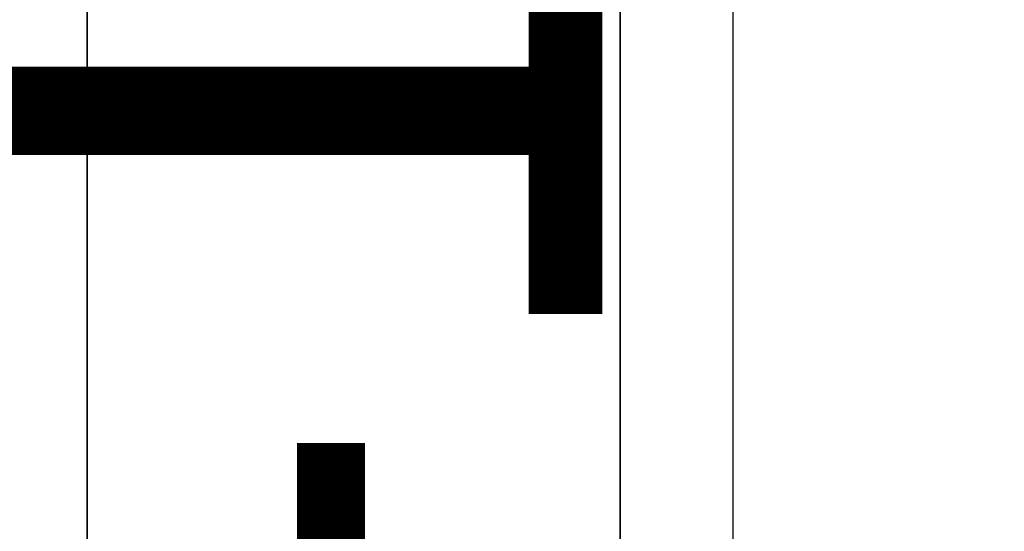
# Model space of a CAD drawing. Units: inches. Extents: x 2083 to 3317, y 1141 to 2115.
# Tile 76 of 256: x 2225.82 to 2242.45, y 1485.75 to 1494.39. Entities that reach past the tile are written whole.
import ezdxf

# ---------------------------------------------------------------- set-up
doc = ezdxf.new("R2010")
doc.units = ezdxf.units.IN
doc.layers.add('A-ANNO-DIMS', color=2, linetype='Continuous', lineweight=18)
doc.layers.add('A-WALL', color=7, linetype='Continuous', lineweight=35)
doc.layers.add('A-WALL-PATT', color=251, linetype='Continuous', lineweight=13, true_color=0x636466)
doc.styles.get("Standard").update_dxf_attribs({"font": 'arial.ttf'})
doc.dimstyles.new('ISO-25', dxfattribs={"dimtxt": 12, "dimasz": 12, "dimexe": 1.25, "dimexo": 0.625, "dimtad": 1, "dimlunit": 3, "dimtxsty": 'Standard', "dimcen": 2.5, "dimadec": 0, "dimazin": 0, "dimtfac": 1, "dimtmove": 0, "dimatfit": 3, "dimfxl": 1, "dimarcsym": 0})

# ---------------------------------------------------------------- blocks, each defined once
blk = doc.blocks.new('*D30')
at = {"layer": 'A-ANNO-DIMS', "color": 0, "lineweight": -2, "transparency": 16777216}
for p, q in [((2240.018, 1445.274), (2240.018, 1448.046)), ((2254.329, 1445.274), (2254.329, 1448.046)), ((2228.018, 1446.796), (2216.018, 1446.796)), ((2240.018, 1446.796), (2254.329, 1446.796)), ((2266.329, 1446.796), (2413.765, 1446.796))]:
    blk.add_line(p, q, dxfattribs=at)
at = {"layer": 'A-ANNO-DIMS', "color": 0, "transparency": 16777216}
for points in [[(2228.018, 1448.796), (2228.018, 1444.796), (2240.018, 1446.796)], [(2266.329, 1448.796), (2266.329, 1444.796), (2254.329, 1446.796)]]:
    blk.add_solid(points, dxfattribs=at)
at = {"layer": 'Defpoints', "color": 0, "transparency": 16777216}
for p in [(2254.329, 1446.796), (2240.018, 1444.649), (2254.329, 1444.649)]:
    blk.add_point(p, dxfattribs=at)
at = {"layer": 'A-ANNO-DIMS', "color": 0, "transparency": 16777216, "insert": (2346.047, 1453.625), "char_height": 12, "attachment_point": 5}
blk.add_mtext('WC 1\'-2 1/2" TYP.', dxfattribs=at)
blk = doc.blocks.new('*D31')
at = {"layer": 'A-ANNO-DIMS', "color": 0, "lineweight": -2, "transparency": 16777216}
for p, q in [((2237.871, 1456.649), (2237.871, 1541.915)), ((2239.393, 1444.649), (2236.621, 1444.649)), ((2237.871, 1431.548), (2237.871, 1444.649)), ((2239.393, 1431.548), (2236.621, 1431.548)), ((2237.871, 1419.548), (2237.871, 1407.548))]:
    blk.add_line(p, q, dxfattribs=at)
at = {"layer": 'A-ANNO-DIMS', "color": 0, "transparency": 16777216}
for points in [[(2235.871, 1456.649), (2239.871, 1456.649), (2237.871, 1444.649)], [(2235.871, 1419.548), (2239.871, 1419.548), (2237.871, 1431.548)]]:
    blk.add_solid(points, dxfattribs=at)
at = {"layer": 'Defpoints', "color": 0, "transparency": 16777216}
for p in [(2237.871, 1444.649), (2240.018, 1444.649), (2240.018, 1431.548)]:
    blk.add_point(p, dxfattribs=at)
at = {"layer": 'A-ANNO-DIMS', "color": 0, "transparency": 16777216, "insert": (2231.217, 1505.282), "char_height": 12, "attachment_point": 5, "rotation": 90}
blk.add_mtext('1\'-1" TYP.', dxfattribs=at)
blk = doc.blocks.new('*D45')
at = {"layer": 'A-ANNO-DIMS', "color": 0, "lineweight": -2, "transparency": 16777216}
for p, q in [((2235.96, 1478.386), (2235.96, 1531.361)), ((2418.96, 1478.386), (2418.96, 1531.361)), ((2247.96, 1530.111), (2406.96, 1530.111))]:
    blk.add_line(p, q, dxfattribs=at)
at = {"layer": 'A-ANNO-DIMS', "color": 0, "transparency": 16777216}
for points in [[(2247.96, 1532.111), (2247.96, 1528.111), (2235.96, 1530.111)], [(2406.96, 1532.111), (2406.96, 1528.111), (2418.96, 1530.111)]]:
    blk.add_solid(points, dxfattribs=at)
at = {"layer": 'Defpoints', "color": 0, "transparency": 16777216}
for p in [(2418.96, 1530.111), (2235.96, 1477.761), (2418.96, 1477.761)]:
    blk.add_point(p, dxfattribs=at)
at = {"layer": 'A-ANNO-DIMS', "color": 0, "transparency": 16777216, "insert": (2327.46, 1536.867), "char_height": 12, "attachment_point": 5}
blk.add_mtext('15\'-3"', dxfattribs=at)
blk = doc.blocks.new('*D62')
at = {"layer": 'A-ANNO-DIMS', "color": 0, "lineweight": -2, "transparency": 16777216}
for p, q in [((2235.96, 1469.386), (2235.96, 1522.361)), ((2379.96, 1469.386), (2379.96, 1522.361)), ((2247.96, 1521.111), (2367.96, 1521.111))]:
    blk.add_line(p, q, dxfattribs=at)
at = {"layer": 'A-ANNO-DIMS', "color": 0, "transparency": 16777216}
for points in [[(2247.96, 1523.111), (2247.96, 1519.111), (2235.96, 1521.111)], [(2367.96, 1523.111), (2367.96, 1519.111), (2379.96, 1521.111)]]:
    blk.add_solid(points, dxfattribs=at)
at = {"layer": 'Defpoints', "color": 0, "transparency": 16777216}
for p in [(2379.96, 1521.111), (2235.96, 1468.761), (2379.96, 1468.761)]:
    blk.add_point(p, dxfattribs=at)
at = {"layer": 'A-ANNO-DIMS', "color": 0, "transparency": 16777216, "insert": (2307.96, 1527.863), "char_height": 12, "attachment_point": 5}
blk.add_mtext('12\'-0"', dxfattribs=at)
blk = doc.blocks.new('*D64')
at = {"layer": 'A-ANNO-DIMS', "color": 0, "lineweight": -2, "transparency": 16777216}
for p, q in [((2236.585, 1702.761), (2289.56, 1702.761)), ((2288.31, 1690.761), (2288.31, 1489.761)), ((2236.585, 1477.761), (2289.56, 1477.761))]:
    blk.add_line(p, q, dxfattribs=at)
at = {"layer": 'A-ANNO-DIMS', "color": 0, "transparency": 16777216}
for points in [[(2286.31, 1690.761), (2290.31, 1690.761), (2288.31, 1702.761)], [(2286.31, 1489.761), (2290.31, 1489.761), (2288.31, 1477.761)]]:
    blk.add_solid(points, dxfattribs=at)
at = {"layer": 'Defpoints', "color": 0, "transparency": 16777216}
for p in [(2235.96, 1702.761), (2235.96, 1477.761), (2288.31, 1477.761)]:
    blk.add_point(p, dxfattribs=at)
at = {"layer": 'A-ANNO-DIMS', "color": 0, "transparency": 16777216, "insert": (2281.558, 1590.261), "char_height": 12, "attachment_point": 5, "rotation": 90}
blk.add_mtext('18\'-9"', dxfattribs=at)

msp = doc.modelspace()

# ---------------------------------------------------------------- hatches: boundary and pattern name
at = {"layer": 'A-WALL-PATT'}
h = msp.add_hatch(color=256, dxfattribs=at)
h.dxf.hatch_style = 1
h.paths.add_polyline_path([(3126.96, 2020.761), (2748.96, 2020.761), (2604.96, 2020.761), (2226.96, 2020.761), (2226.96, 1702.761), (2466.96, 1702.761), (2466.96, 1582.761), (2418.96, 1582.761), (2418.96, 1477.761), (2226.96, 1477.761), (2226.96, 1263.261), (2544.96, 1263.261), (2544.96, 1411.761), (2604.96, 1411.761), (2685.96, 1411.761), (2685.96, 1420.761), (2604.96, 1420.761), (2604.96, 1573.761), (2604.96, 1702.761), (2604.96, 2011.761), (2748.96, 2011.761), (2748.96, 1702.761), (2862.96, 1702.761), (2862.96, 1621.761), (2871.96, 1621.761), (2871.96, 1702.761), (2883.96, 1702.761), (2883.96, 1706.939, -0.026459), (2883.96, 1711.761), (2757.96, 1711.761), (2757.96, 1807.761), (2787.96, 1807.761), (2787.96, 1812.261), (2757.96, 1812.261), (2757.96, 2011.761), (2877.96, 2011.761), (2877.96, 1812.261), (2847.96, 1812.261), (2847.96, 1807.761), (2889.836, 1807.761), (2889.836, 1812.261), (2882.46, 1812.261), (2882.46, 2011.761), (3117.96, 2011.761), (3117.96, 1812.261), (2937.836, 1812.261), (2937.836, 1807.761), (2995.71, 1807.761), (2995.71, 1796.118), (3000.21, 1796.118), (3000.21, 1807.761), (3117.96, 1807.761), (3117.96, 1711.761), (3000.21, 1711.761), (3000.21, 1760.118), (2998.573, 1760.118, -0.020711), (2995.71, 1760.118), (2995.71, 1711.761), (2931.96, 1711.761), (2931.96, 1702.761), (3126.96, 1702.761)])
h.paths.add_polyline_path([(2471.46, 2011.761), (2471.46, 1810.011), (2462.717, 1810.011), (2462.717, 1805.511), (2505.96, 1805.511), (2505.96, 1810.011), (2475.96, 1810.011), (2475.96, 2011.761), (2595.96, 2011.761), (2595.96, 1810.011), (2565.96, 1810.011), (2565.96, 1805.511), (2595.96, 1805.511), (2595.96, 1711.761), (2235.96, 1711.761), (2235.96, 1805.511), (2353.71, 1805.511), (2353.71, 1796.054), (2358.21, 1796.054), (2358.21, 1805.511), (2414.717, 1805.511), (2414.717, 1810.011), (2235.96, 1810.011), (2235.96, 2011.761)], flags=16)
h.paths.add_polyline_path([(2270.205, 1994.61), (2270.205, 1970.61), (2246.205, 1970.61), (2246.205, 1994.61)], flags=0)
edge = h.paths.add_edge_path(flags=0)
edge.add_ellipse((2332.027, 1899.798), major_axis=(-3.043, 3.043), ratio=0.168252, start_angle=-161.3322, end_angle=-156.3071, ccw=False)
edge.add_ellipse((2333.082, 1898.744), major_axis=(-1.055, 1.055), ratio=0.453532, start_angle=-123.371, end_angle=-94.1591)
edge = h.paths.add_edge_path(flags=0)
edge.add_ellipse((2332.027, 1968.876), major_axis=(3.043, 3.043), ratio=0.168252, start_angle=18.6678, end_angle=23.6929)
edge.add_spline(control_points=[(2332.926, 1970.691), (2332.227, 1970.336), (2330.894, 1969.659), (2328.413, 1970.932), (2327.204, 1967.749), (2324.71, 1969.956), (2322.533, 1967.012), (2320.013, 1971.296), (2317.68, 1968.158), (2316.041, 1967.102), (2315.427, 1966.81)], knot_values=[0, 0, 0, 0, 2.267059, 4.324559, 6.685584, 8.878641, 11.121502, 14.300359, 17.755284, 19.732645, 19.732645, 19.732645, 19.732645], degree=3, periodic=0)
edge.add_ellipse((2332.027, 1968.876), major_axis=(3.043, 3.043), ratio=0.168252, start_angle=18.6678, end_angle=23.6929, ccw=False)
edge.add_ellipse((2333.082, 1969.931), major_axis=(1.055, 1.055), ratio=0.453532, start_angle=56.629, end_angle=85.8409, ccw=False)
edge = h.paths.add_edge_path(flags=0)
edge.add_spline(control_points=[(2296.428, 1967.988), (2293.628, 1965.336), (2287.704, 1959.727), (2299.744, 1949.996), (2294.533, 1935.669), (2290.573, 1920.604), (2293.394, 1909.974), (2296.185, 1904.967)], knot_values=[0.099185, 0.099185, 0.099185, 0.099185, 0.345301, 0.619822, 0.982653, 1.386093, 1.810555, 1.810555, 1.810555, 1.810555], degree=3, periodic=0)
edge.add_spline(control_points=[(2296.185, 1904.967), (2297.384, 1902.619), (2298.001, 1901.949), (2298.553, 1901.468)], knot_values=[0.006246, 0.006246, 0.006246, 0.006246, 0.055476, 0.055476, 0.055476, 0.055476], degree=3, periodic=0)
edge.add_spline(control_points=[(2298.553, 1901.468), (2297.259, 1900.923), (2295.225, 1900.232), (2293.06, 1900.614), (2292.101, 1900.788), (2292.09, 1900.791)], knot_values=[0.312835, 0.312835, 0.312835, 0.312835, 0.40178, 0.474987, 0.475903, 0.475903, 0.475903, 0.475903], degree=3, periodic=0)
edge.add_arc((2292.794, 1904.664), 3.937, 215.4209, 259.6982, ccw=False)
edge.add_spline(control_points=[(2289.585, 1902.382), (2289.477, 1902.535), (2289.368, 1902.688), (2289.261, 1902.841)], knot_values=[0.102872, 0.102872, 0.102872, 0.102872, 0.116896, 0.116896, 0.116896, 0.116896], degree=3, periodic=0)
edge.add_spline(control_points=[(2289.261, 1902.841), (2288.687, 1902.55), (2287.64, 1902.02), (2285.881, 1901.874), (2283.853, 1901.504), (2281.72, 1899.711), (2278.467, 1899.493), (2276.157, 1901.883), (2272.259, 1899.804), (2267.778, 1901.843), (2262.244, 1900.184), (2257.415, 1901.782), (2254.318, 1900.726), (2253.178, 1900.337)], knot_values=[0, 0, 0, 0, 1.907977, 3.477176, 5.261074, 7.972851, 11.680248, 13.717921, 16.939592, 22.789562, 27.502503, 33.595215, 37.145618, 37.145618, 37.145618, 37.145618], degree=3, periodic=0)
edge.add_line((2253.178, 1900.337), (2250.244, 1902.841))
edge.add_line((2250.244, 1902.841), (2250.244, 1965.833))
edge.add_line((2250.244, 1965.833), (2253.178, 1968.337))
edge.add_spline(control_points=[(2253.178, 1968.337), (2254.318, 1967.948), (2257.415, 1966.892), (2262.244, 1968.49), (2267.778, 1966.831), (2271.527, 1968.537), (2273.876, 1967.828), (2274.207, 1967.728)], knot_values=[0, 0, 0, 0, 0.09018, 0.244935, 0.364644, 0.513233, 0.537855, 0.537855, 0.537855, 0.537855], degree=3, periodic=0)
edge.add_arc((2274.353, 1963.793), 3.937, 72.0511, 92.1279, ccw=False)
edge.add_arc((2281.297, 1985.23), 18.596, 252.0511, 288.5657)
edge.add_arc((2292.317, 1956.029), 12.646, 71.0268, 113.7782, ccw=False)
edge = h.paths.add_edge_path(flags=0)
edge.add_spline(control_points=[(2274.899, 1951.856), (2275.066, 1951.617), (2275.233, 1951.377), (2275.398, 1951.136)], knot_values=[1.409916, 1.409916, 1.409916, 1.409916, 1.43159, 1.43159, 1.43159, 1.43159], degree=3, periodic=0)
edge.add_spline(control_points=[(2275.398, 1951.136), (2275.792, 1950.562), (2276.179, 1949.984), (2276.546, 1949.397)], knot_values=[1.358238, 1.358238, 1.358238, 1.358238, 1.409916, 1.409916, 1.409916, 1.409916], degree=3, periodic=0)
edge.add_line((2276.546, 1949.397), (2277.437, 1947.862))
edge.add_spline(control_points=[(2277.437, 1947.862), (2276.304, 1945.673), (2274.64, 1942.427), (2274.632, 1938.094), (2272.799, 1930.852), (2274.356, 1943.897), (2275.948, 1947.923), (2276.546, 1949.397)], knot_values=[0.005632, 0.005632, 0.005632, 0.005632, 0.186014, 0.266002, 0.357087, 0.59639, 0.739732, 0.739732, 0.739732, 0.739732], degree=3, periodic=0)
edge.add_spline(control_points=[(2276.546, 1949.397), (2276.179, 1949.984), (2275.792, 1950.562), (2275.398, 1951.136)], knot_values=[1.358238, 1.358238, 1.358238, 1.358238, 1.409916, 1.409916, 1.409916, 1.409916], degree=3, periodic=0)
edge.add_spline(control_points=[(2275.398, 1951.136), (2274.943, 1950.08), (2274.208, 1948.025), (2273.935, 1944.851), (2272.469, 1937.627), (2273.466, 1945.696), (2274.701, 1951.059), (2274.899, 1951.856)], knot_values=[0.104364, 0.104364, 0.104364, 0.104364, 0.189636, 0.269624, 0.36071, 0.600013, 0.644622, 0.644622, 0.644622, 0.644622], degree=3, periodic=0)
h.paths.add_polyline_path([(2269.168, 1963.128, -0.357527), (2268.171, 1960.976, -0.092561), (2268.171, 1939.436, -0.357527), (2269.168, 1937.285, -0.357527), (2267.016, 1938.282, -0.164785), (2254.686, 1938.282, -0.357527), (2252.534, 1937.285, -0.357527), (2253.531, 1939.436, -0.092561), (2253.531, 1960.976, -0.357527), (2252.534, 1963.128, -0.357527), (2254.686, 1962.131, -0.164785), (2267.016, 1962.131, -0.357527)], flags=0)
h.paths.add_polyline_path([(2248.874, 1967.802), (2248.874, 1957.028), (2249.458, 1957.028), (2249.458, 1911.647), (2248.874, 1911.647), (2248.874, 1900.873), (2246.512, 1900.873, 0.197327), (2244.15, 1902.457), (2244.15, 1966.218, 0.197327), (2246.512, 1967.802)], flags=0)
h.paths.add_polyline_path([(2269.168, 1931.389, -0.357527), (2268.171, 1929.238, -0.092561), (2268.171, 1907.698, -0.357527), (2269.168, 1905.547, -0.357527), (2267.016, 1906.544, -0.164785), (2254.686, 1906.544, -0.357527), (2252.534, 1905.547, -0.357527), (2253.531, 1907.698, -0.092561), (2253.531, 1929.238, -0.357527), (2252.534, 1931.389, -0.357527), (2254.686, 1930.392, -0.164785), (2267.016, 1930.392, -0.357527)], flags=0)
edge = h.paths.add_edge_path(flags=0)
edge.add_spline(control_points=[(2276.197, 1906.724), (2276.168, 1909.029), (2276.114, 1913.372), (2270.598, 1924.925), (2273.905, 1919.013), (2275.922, 1916.262), (2275.475, 1912.402), (2277.258, 1910.381), (2276.696, 1908.225), (2276.646, 1906.813), (2276.618, 1906.008)], knot_values=[0, 0, 0, 0, 8.61026, 16.221274, 18.843057, 23.804898, 27.440828, 29.356102, 31.203478, 33.650687, 33.650687, 33.650687, 33.650687], degree=3, periodic=0)
edge.add_spline(control_points=[(2276.618, 1906.008), (2276.623, 1905.624), (2276.498, 1904.629), (2275.442, 1903.855), (2274.937, 1903.08), (2274.859, 1902.841)], knot_values=[0.156488, 0.156488, 0.156488, 0.156488, 0.184398, 0.231376, 0.250598, 0.250598, 0.250598, 0.250598], degree=3, periodic=0)
edge.add_line((2274.859, 1902.841), (2276.506, 1902.841))
edge.add_spline(control_points=[(2276.506, 1902.841), (2276.788, 1903.085), (2277.665, 1904.125), (2278.25, 1904.341), (2277.654, 1908.527), (2278.156, 1906.228), (2278.1, 1905.286), (2278.847, 1904.069), (2277.857, 1903.415), (2277.874, 1902.991), (2277.904, 1902.841)], knot_values=[0.059574, 0.059574, 0.059574, 0.059574, 0.080753, 0.103741, 0.16972, 0.176036, 0.207137, 0.240474, 0.262341, 0.27366, 0.27366, 0.27366, 0.27366], degree=3, periodic=0)
edge.add_line((2277.904, 1902.841), (2280.03, 1902.841))
edge.add_spline(control_points=[(2280.03, 1902.841), (2279.888, 1903.088), (2279.499, 1903.982), (2280.152, 1905.939), (2278.104, 1909.658), (2279.762, 1907.185), (2280.328, 1904.875), (2280.485, 1903.49), (2281.463, 1903.249), (2281.758, 1902.936), (2281.834, 1902.841)], knot_values=[0.013856, 0.013856, 0.013856, 0.013856, 0.034874, 0.088867, 0.107879, 0.126738, 0.158714, 0.193757, 0.217487, 0.226722, 0.226722, 0.226722, 0.226722], degree=3, periodic=0)
edge.add_spline(control_points=[(2281.834, 1902.841), (2281.788, 1902.827), (2281.647, 1902.783), (2281.396, 1902.859), (2281.088, 1902.985), (2280.721, 1903.061), (2280.333, 1903.026), (2280.125, 1902.899), (2280.03, 1902.841)], knot_values=[0, 0, 0, 0, 0.14413, 0.435517, 0.749276, 1.153046, 1.548371, 1.878348, 1.878348, 1.878348, 1.878348], degree=3, periodic=0)
edge.add_line((2280.03, 1902.841), (2277.904, 1902.841))
edge.add_spline(control_points=[(2277.904, 1902.841), (2277.893, 1902.796), (2277.865, 1902.68), (2277.607, 1902.687), (2277.274, 1902.801), (2276.838, 1902.62), (2276.584, 1902.789), (2276.506, 1902.841)], knot_values=[0, 0, 0, 0, 0.127189, 0.326199, 0.628009, 1.24357, 1.515331, 1.515331, 1.515331, 1.515331], degree=3, periodic=0)
edge.add_line((2276.506, 1902.841), (2274.859, 1902.841))
edge.add_spline(control_points=[(2274.859, 1902.841), (2274.814, 1902.899), (2274.725, 1903.013), (2274.493, 1903.119), (2274.244, 1902.961), (2273.937, 1903.185), (2273.614, 1902.983), (2273.408, 1902.883), (2273.322, 1902.841)], knot_values=[0, 0, 0, 0, 0.21843, 0.436957, 0.687977, 0.990379, 1.398396, 1.69185, 1.69185, 1.69185, 1.69185], degree=3, periodic=0)
edge.add_spline(control_points=[(2273.322, 1902.841), (2273.617, 1903.446), (2274.274, 1904.538), (2276.027, 1904.574), (2276.207, 1906.584), (2276.197, 1906.724)], knot_values=[0.012227, 0.012227, 0.012227, 0.012227, 0.059472, 0.106218, 0.134458, 0.134458, 0.134458, 0.134458], degree=3, periodic=0)
h.paths.add_polyline_path([(2270.776, 1897.79), (2270.776, 1873.79), (2246.776, 1873.79), (2246.776, 1897.79)], flags=0)
h.paths.add_polyline_path([(2353.71, 1760.005), (2353.71, 1760.054), (2358.21, 1760.054, -0.033729)], flags=0)
h.paths.add_polyline_path([(2321.819, 1737.529), (2341.995, 1737.529, -0.414214), (2343.203, 1736.321), (2343.203, 1721.021, -0.414214), (2341.995, 1719.813), (2321.819, 1719.813, -0.414214), (2320.611, 1721.021), (2320.611, 1736.321, -0.414214)], flags=0)
h.paths.add_polyline_path([(2324.235, 1736.321), (2339.579, 1736.321, -0.414214), (2341.995, 1733.905), (2341.995, 1725.45, -0.414214), (2339.579, 1723.034), (2333.681, 1723.034), (2333.845, 1722.045, -0.870646), (2335.425, 1721.826, -0.767327), (2333.923, 1721.423), (2331.291, 1721.423, -0.767327), (2329.788, 1721.826, -0.870646), (2331.368, 1722.045), (2331.533, 1723.034), (2324.235, 1723.034, -0.414214), (2321.819, 1725.45), (2321.819, 1733.905, -0.414214)], flags=0)
h.paths.add_polyline_path([(2570.484, 1928.615), (2589.684, 1928.615), (2590.169, 1928.615), (2590.169, 1904.993), (2570.484, 1904.993)], flags=0)
h.paths.add_polyline_path([(2574.447, 1927.264, -1), (2572.829, 1927.264, -1)], flags=0)
h.paths.add_polyline_path([(2573.09, 1926.941), (2573.925, 1927.776), (2574.148, 1927.553), (2573.313, 1926.718)], flags=0)
h.paths.add_polyline_path([(2578.779, 1919.73, -1), (2571.592, 1919.73, -1)], flags=0)
h.paths.add_polyline_path([(2578.385, 1919.73, -1), (2571.985, 1919.73, -1)], flags=0)
h.paths.add_polyline_path([(2331.596, 1729.476, -1), (2333.618, 1729.476, -1)], flags=0)
h.paths.add_polyline_path([(2578.034, 1927.264, -1), (2576.416, 1927.264, -1)], flags=0)
h.paths.add_polyline_path([(2576.689, 1927.531), (2576.912, 1927.754), (2577.747, 1926.919), (2577.524, 1926.696)], flags=0)
h.paths.add_polyline_path([(2578.139, 1909.86, -1), (2572.232, 1909.86, -1)], flags=0)
h.paths.add_polyline_path([(2577.745, 1909.86, -1), (2572.625, 1909.86, -1)], flags=0)
h.paths.add_polyline_path([(2583.798, 1927.264, -1), (2582.179, 1927.264, -1)], flags=0)
h.paths.add_polyline_path([(2582.719, 1927.754), (2583.554, 1926.919), (2583.331, 1926.696), (2582.496, 1927.531)], flags=0)
h.paths.add_polyline_path([(2582.496, 1927.531), (2582.719, 1927.754), (2583.554, 1926.919), (2583.331, 1926.696)], flags=0)
h.paths.add_polyline_path([(2587.739, 1920.53, -1), (2581.832, 1920.53, -1)], flags=0)
h.paths.add_polyline_path([(2587.345, 1920.53, -1), (2582.225, 1920.53, -1)], flags=0)
h.paths.add_polyline_path([(2587.385, 1927.264, -1), (2585.766, 1927.264, -1)], flags=0)
h.paths.add_polyline_path([(2586.082, 1926.98), (2586.917, 1927.815), (2587.14, 1927.593), (2586.305, 1926.758)], flags=0)
h.paths.add_polyline_path([(2588.379, 1910.66, -1), (2581.192, 1910.66, -1)], flags=0)
h.paths.add_polyline_path([(2587.985, 1910.66, -1), (2581.585, 1910.66, -1)], flags=0)
h.paths.add_polyline_path([(2417.168, 1729.478), (2437.344, 1729.478, -0.414214), (2438.552, 1728.27), (2438.552, 1712.969, -0.414214), (2437.344, 1711.761), (2417.168, 1711.761, -0.414214), (2415.96, 1712.969), (2415.96, 1728.27, -0.414214)], flags=0)
h.paths.add_polyline_path([(2419.584, 1728.27), (2434.928, 1728.27, -0.414214), (2437.344, 1725.854), (2437.344, 1717.398, -0.414214), (2434.928, 1714.983), (2429.029, 1714.983), (2429.194, 1713.994, -0.870646), (2430.774, 1713.775, -0.767327), (2429.271, 1713.372), (2426.64, 1713.372, -0.767327), (2425.137, 1713.775, -0.870646), (2426.717, 1713.994), (2426.882, 1714.983), (2419.584, 1714.983, -0.414214), (2417.168, 1717.398), (2417.168, 1725.854, -0.414214)], flags=0)
h.paths.add_polyline_path([(2419.584, 1728.27), (2434.928, 1728.27, -0.414214), (2437.344, 1725.854), (2437.344, 1717.398, -0.414214), (2434.928, 1714.983), (2429.029, 1714.983), (2428.358, 1719.009), (2427.553, 1719.009), (2426.882, 1714.983), (2419.584, 1714.983, -0.414214), (2417.168, 1717.398), (2417.168, 1725.854, -0.414214)], flags=0)
h.paths.add_polyline_path([(2426.944, 1721.425, -1), (2428.967, 1721.425, -1)], flags=0)
h.paths.add_polyline_path([(2475.96, 1702.761), (2595.96, 1702.761), (2595.96, 1582.761), (2475.96, 1582.761)], flags=16)
h.paths.add_polyline_path([(2427.96, 1573.761), (2595.96, 1573.761), (2595.96, 1468.761), (2595.96, 1420.761), (2384.46, 1420.761), (2384.46, 1468.761), (2427.96, 1468.761)], flags=16)
h.paths.add_polyline_path([(2379.96, 1468.761), (2379.96, 1420.761), (2235.96, 1420.761), (2235.96, 1468.761)], flags=16)
h.paths.add_polyline_path([(2317.816, 1466.696), (2337.992, 1466.696, -0.414214), (2339.2, 1465.488), (2339.2, 1450.187, -0.414214), (2337.992, 1448.979), (2317.816, 1448.979, -0.414214), (2316.608, 1450.187), (2316.608, 1465.488, -0.414214)], flags=0)
h.paths.add_polyline_path([(2320.232, 1465.488), (2335.576, 1465.488, -0.414214), (2337.992, 1463.072), (2337.992, 1454.616, -0.414214), (2335.576, 1452.2), (2329.677, 1452.2), (2329.842, 1451.212, -0.870646), (2331.422, 1450.992, -0.767327), (2329.92, 1450.59), (2327.288, 1450.59, -0.767327), (2325.785, 1450.992, -0.870646), (2327.365, 1451.212), (2327.53, 1452.2), (2320.232, 1452.2, -0.414214), (2317.816, 1454.616), (2317.816, 1463.072, -0.414214)], flags=0)
h.paths.add_polyline_path([(2320.232, 1465.488), (2335.576, 1465.488, -0.414214), (2337.992, 1463.072), (2337.992, 1454.616, -0.414214), (2335.576, 1452.2), (2329.677, 1452.2), (2329.006, 1456.227), (2328.201, 1456.227), (2327.53, 1452.2), (2320.232, 1452.2, -0.414214), (2317.816, 1454.616), (2317.816, 1463.072, -0.414214)], flags=0)
h.paths.add_polyline_path([(2327.593, 1458.643, -1), (2329.615, 1458.643, -1)], flags=0)
h.paths.add_polyline_path([(2244.412, 1433.34), (2241.921, 1433.34, -0.414214), (2240.018, 1435.244), (2240.018, 1440.953, -0.414211), (2241.921, 1442.856), (2244.412, 1442.856, -1.976472)], flags=0)
h.paths.add_polyline_path([(2245.357, 1434.398, -0.414214), (2245.357, 1441.799, -2.144098)], flags=0)
h.paths.add_polyline_path([(2535.96, 1416.261), (2535.96, 1272.261), (2235.96, 1272.261), (2235.96, 1416.261)], flags=16)
h.paths.add_polyline_path([(2260.12, 1384.293), (2260.12, 1362.039), (2237.865, 1362.039), (2237.865, 1384.293)], flags=0)
edge = h.paths.add_edge_path(flags=0)
edge.add_line((2318.252, 1362.093), (2318.146, 1362.001))
edge.add_ellipse((2317.445, 1360.431), major_axis=(2.822, 2.822), ratio=0.168252, start_angle=18.6678, end_angle=20.9481, ccw=False)
edge.add_ellipse((2318.423, 1361.409), major_axis=(0.978, 0.978), ratio=0.453532, start_angle=56.629, end_angle=70.2262, ccw=False)
edge = h.paths.add_edge_path(flags=0)
edge.add_line((2319.107, 1295.571), (2319.015, 1295.677))
edge.add_ellipse((2317.445, 1296.378), major_axis=(-2.822, 2.822), ratio=0.168252, start_angle=-161.3322, end_angle=-159.0519, ccw=False)
edge.add_ellipse((2318.423, 1295.4), major_axis=(-0.978, 0.978), ratio=0.453532, start_angle=-123.371, end_angle=-109.7738)
edge = h.paths.add_edge_path(flags=0)
edge.add_spline(control_points=[(2284.21, 1301.17), (2284.581, 1300.445), (2284.891, 1299.892), (2285.16, 1299.461)], knot_values=[0.039066, 0.039066, 0.039066, 0.039066, 0.055476, 0.055476, 0.055476, 0.055476], degree=3, periodic=0)
edge.add_line((2285.16, 1299.461), (2284.21, 1301.17))
edge = h.paths.add_edge_path(flags=0)
edge.add_line((2280.412, 1297.298), (2283.37, 1297.036))
edge.add_line((2283.37, 1297.036), (2286.406, 1297.926))
edge.add_spline(control_points=[(2286.406, 1297.926), (2285.305, 1297.463), (2284.345, 1297.129), (2283.37, 1297.036)], knot_values=[0.394369, 0.394369, 0.394369, 0.394369, 0.475903, 0.475903, 0.475903, 0.475903], degree=3, periodic=0)
edge.add_spline(control_points=[(2283.37, 1297.036), (2283.281, 1297.028), (2282.316, 1296.957), (2281.313, 1297.134), (2280.423, 1297.296), (2280.412, 1297.298)], knot_values=[0.312835, 0.312835, 0.312835, 0.312835, 0.320246, 0.393453, 0.394369, 0.394369, 0.394369, 0.394369], degree=3, periodic=0)
edge = h.paths.add_edge_path(flags=0)
edge.add_line((2284.436, 1359.607), (2280.446, 1355.328))
edge.add_line((2280.446, 1355.328), (2279.58, 1351.018))
edge.add_line((2279.58, 1351.018), (2282.413, 1346.58))
edge.add_spline(control_points=[(2282.413, 1346.58), (2283.153, 1345.589), (2284.253, 1344.029), (2284.801, 1342.387), (2284.935, 1341.806)], knot_values=[1.240098, 1.240098, 1.240098, 1.240098, 1.332892, 1.382712, 1.382712, 1.382712, 1.382712], degree=3, periodic=0)
edge.add_spline(control_points=[(2284.935, 1341.806), (2285.319, 1340.141), (2285.233, 1338.409), (2284.91, 1336.654)], knot_values=[1.097484, 1.097484, 1.097484, 1.097484, 1.240098, 1.240098, 1.240098, 1.240098], degree=3, periodic=0)
edge.add_spline(control_points=[(2284.91, 1336.654), (2284.587, 1334.899), (2284.027, 1333.12), (2283.463, 1331.361)], knot_values=[0.95487, 0.95487, 0.95487, 0.95487, 1.097484, 1.097484, 1.097484, 1.097484], degree=3, periodic=0)
edge.add_line((2283.463, 1331.361), (2281.89, 1326.153))
edge.add_line((2281.89, 1326.153), (2280.756, 1321.056))
edge.add_line((2280.756, 1321.056), (2280.299, 1316.002))
edge.add_line((2280.299, 1316.002), (2280.716, 1310.95))
edge.add_line((2280.716, 1310.95), (2282.028, 1305.972))
edge.add_line((2282.028, 1305.972), (2284.21, 1301.17))
edge.add_spline(control_points=[(2284.21, 1301.17), (2283.341, 1302.73), (2282.612, 1304.336), (2282.028, 1305.972)], knot_values=[0.099185, 0.099185, 0.099185, 0.099185, 0.241799, 0.241799, 0.241799, 0.241799], degree=3, periodic=0)
edge.add_spline(control_points=[(2282.028, 1305.972), (2281.444, 1307.608), (2281.005, 1309.273), (2280.716, 1310.95)], knot_values=[0.241799, 0.241799, 0.241799, 0.241799, 0.384413, 0.384413, 0.384413, 0.384413], degree=3, periodic=0)
edge.add_spline(control_points=[(2280.716, 1310.95), (2280.433, 1312.588), (2280.289, 1314.277), (2280.299, 1315.962), (2280.299, 1316.002)], knot_values=[0.384413, 0.384413, 0.384413, 0.384413, 0.523647, 0.527028, 0.527028, 0.527028, 0.527028], degree=3, periodic=0)
edge.add_spline(control_points=[(2280.299, 1316.002), (2280.312, 1317.687), (2280.478, 1319.368), (2280.756, 1321.056)], knot_values=[0.527028, 0.527028, 0.527028, 0.527028, 0.669642, 0.669642, 0.669642, 0.669642], degree=3, periodic=0)
edge.add_spline(control_points=[(2280.756, 1321.056), (2281.035, 1322.744), (2281.426, 1324.44), (2281.89, 1326.153)], knot_values=[0.669642, 0.669642, 0.669642, 0.669642, 0.812256, 0.812256, 0.812256, 0.812256], degree=3, periodic=0)
edge.add_spline(control_points=[(2281.89, 1326.153), (2282.264, 1327.533), (2282.788, 1329.262), (2283.353, 1331.018), (2283.463, 1331.361)], knot_values=[0.812256, 0.812256, 0.812256, 0.812256, 0.927087, 0.95487, 0.95487, 0.95487, 0.95487], degree=3, periodic=0)
edge.add_line((2283.463, 1331.361), (2284.91, 1336.654))
edge.add_line((2284.91, 1336.654), (2284.935, 1341.806))
edge.add_line((2284.935, 1341.806), (2282.413, 1346.58))
edge.add_spline(control_points=[(2282.413, 1346.58), (2281.275, 1348.104), (2280.078, 1349.57), (2279.58, 1351.018)], knot_values=[1.382712, 1.382712, 1.382712, 1.382712, 1.525326, 1.525326, 1.525326, 1.525326], degree=3, periodic=0)
edge.add_spline(control_points=[(2279.58, 1351.018), (2279.443, 1351.415), (2279.136, 1352.857), (2279.735, 1354.29), (2280.446, 1355.328)], knot_values=[1.525326, 1.525326, 1.525326, 1.525326, 1.564439, 1.667941, 1.667941, 1.667941, 1.667941], degree=3, periodic=0)
edge.add_spline(control_points=[(2280.446, 1355.328), (2281.426, 1356.758), (2282.931, 1358.183), (2284.436, 1359.607)], knot_values=[1.667941, 1.667941, 1.667941, 1.667941, 1.810555, 1.810555, 1.810555, 1.810555], degree=3, periodic=0)
edge.add_arc((2280.623, 1348.518), 11.726, 71.0268, 113.7782)
edge.add_arc((2270.405, 1375.595), 17.244, 252.0511, 288.5657, ccw=False)
edge.add_arc((2263.966, 1355.718), 3.651, 72.0511, 92.1279)
edge.add_arc((2263.966, 1355.718), 3.651, 92.1279, 177.9851)
edge.add_spline(control_points=[(2260.318, 1355.846), (2260.26, 1354.221), (2260.551, 1350.187), (2262.999, 1346.766), (2264.473, 1344.649)], knot_values=[1.43159, 1.43159, 1.43159, 1.43159, 1.564144, 1.770695, 1.770695, 1.770695, 1.770695], degree=3, periodic=0)
edge.add_line((2264.473, 1344.649), (2264.936, 1343.983))
edge.add_spline(control_points=[(2263.801, 1340.248), (2263.843, 1340.514), (2264.067, 1341.756), (2264.513, 1343.002), (2264.935, 1343.981)], knot_values=[0.53657, 0.53657, 0.53657, 0.53657, 0.559349, 0.644622, 0.644622, 0.644622, 0.644622], degree=3, periodic=0)
edge.add_spline(control_points=[(2264.935, 1343.981), (2265.118, 1343.715), (2265.299, 1343.448), (2265.477, 1343.179)], knot_values=[1.384077, 1.384077, 1.384077, 1.384077, 1.409916, 1.409916, 1.409916, 1.409916], degree=3, periodic=0)
edge.add_spline(control_points=[(2265.477, 1343.179), (2265.655, 1342.911), (2265.829, 1342.641), (2265.999, 1342.369)], knot_values=[1.358238, 1.358238, 1.358238, 1.358238, 1.384077, 1.384077, 1.384077, 1.384077], degree=3, periodic=0)
edge.add_line((2265.999, 1342.369), (2266.826, 1340.946))
edge.add_spline(control_points=[(2266.826, 1340.946), (2268.894, 1337.09), (2271.398, 1325.843), (2270.516, 1310.569), (2275.919, 1301.861), (2277.79, 1299.199)], knot_values=[0.116896, 0.116896, 0.116896, 0.116896, 0.472987, 1.050969, 1.313793, 1.313793, 1.313793, 1.313793], degree=3, periodic=0)
edge.add_spline(control_points=[(2277.79, 1299.199), (2277.839, 1299.128), (2277.889, 1299.057), (2277.94, 1298.987)], knot_values=[0.109884, 0.109884, 0.109884, 0.109884, 0.116896, 0.116896, 0.116896, 0.116896], degree=3, periodic=0)
edge.add_line((2277.94, 1298.987), (2277.789, 1299.199))
edge.add_spline(control_points=[(2277.789, 1299.199), (2277.257, 1298.929), (2276.286, 1298.438), (2275.039, 1298.334), (2274.383, 1298.239), (2274.215, 1298.209)], knot_values=[33.12187, 33.12187, 33.12187, 33.12187, 35.029056, 36.598255, 37.144827, 37.144827, 37.144827, 37.144827], degree=3, periodic=0)
edge.add_line((2274.215, 1298.209), (2273.073, 1297.893))
edge.add_spline(control_points=[(2273.073, 1297.893), (2272.323, 1297.58), (2271.039, 1296.511), (2269.248, 1296.226), (2268.423, 1296.375)], knot_values=[26.532584, 26.532584, 26.532584, 26.532584, 29.198919, 31.839101, 31.839101, 31.839101, 31.839101], degree=3, periodic=0)
edge.add_line((2268.423, 1296.375), (2263.879, 1297.458))
edge.add_spline(control_points=[(2263.879, 1297.458), (2263.556, 1297.359), (2261.86, 1296.839), (2260.239, 1297.282), (2258.933, 1297.516)], knot_values=[15.919551, 15.919551, 15.919551, 15.919551, 16.939592, 21.226067, 21.226067, 21.226067, 21.226067], degree=3, periodic=0)
edge.add_line((2258.933, 1297.516), (2254.055, 1297.329))
edge.add_spline(control_points=[(2254.055, 1297.329), (2253.756, 1297.296), (2252.114, 1297.165), (2250.462, 1297.544), (2249.13, 1297.668)], knot_values=[5.306517, 5.306517, 5.306517, 5.306517, 6.276435, 10.613034, 10.613034, 10.613034, 10.613034], degree=3, periodic=0)
edge.add_line((2249.13, 1297.668), (2244.332, 1296.878))
edge.add_line((2244.332, 1296.878), (2241.611, 1299.199))
edge.add_line((2241.611, 1299.199), (2241.611, 1357.609))
edge.add_line((2241.611, 1357.609), (2244.332, 1359.931))
edge.add_line((2244.332, 1359.931), (2252.729, 1359.543))
edge.add_spline(control_points=[(2252.729, 1359.543), (2252.871, 1359.546), (2253.306, 1359.548), (2253.74, 1359.514), (2254.032, 1359.482)], knot_values=[0.233291, 0.233291, 0.233291, 0.233291, 0.244935, 0.268927, 0.268927, 0.268927, 0.268927], degree=3, periodic=0)
edge.add_line((2254.032, 1359.482), (2259.587, 1359.416))
edge.add_spline(control_points=[(2259.587, 1359.416), (2260.677, 1359.629), (2262.073, 1359.897), (2263.524, 1359.459), (2263.83, 1359.366)], knot_values=[0.422516, 0.422516, 0.422516, 0.422516, 0.513233, 0.537855, 0.537855, 0.537855, 0.537855], degree=3, periodic=0)
edge.add_arc((2263.966, 1355.718), 3.651, 72.0511, 92.1279, ccw=False)
edge.add_arc((2270.405, 1375.595), 17.244, 252.0511, 288.5657)
edge.add_arc((2280.623, 1348.518), 11.726, 71.0268, 113.7782, ccw=False)
h.paths.add_polyline_path([(2240.341, 1359.435), (2240.341, 1349.444), (2240.882, 1349.444), (2240.882, 1307.365), (2240.341, 1307.365), (2240.341, 1297.374), (2238.15, 1297.374, 0.197327), (2235.96, 1298.843), (2235.96, 1357.966, 0.197327), (2238.15, 1359.435)], flags=0)
h.paths.add_polyline_path([(2259.158, 1355.101, -0.357527), (2258.233, 1353.106, -0.092561), (2258.233, 1333.133, -0.357527), (2259.158, 1331.138, -0.357527), (2257.163, 1332.062, -0.164785), (2245.729, 1332.062, -0.357527), (2243.735, 1331.138, -0.357527), (2244.659, 1333.133, -0.092561), (2244.659, 1353.106, -0.357527), (2243.735, 1355.101, -0.357527), (2245.729, 1354.176, -0.164785), (2257.163, 1354.176, -0.357527)], flags=0)
edge = h.paths.add_edge_path(flags=0)
edge.add_line((2265.999, 1342.369), (2266.826, 1340.946))
edge.add_line((2266.826, 1340.946), (2265.308, 1337.814))
edge.add_line((2265.308, 1337.814), (2264.358, 1334.653))
edge.add_line((2264.358, 1334.653), (2264.262, 1333.8))
edge.add_spline(control_points=[(2264.262, 1333.8), (2264.208, 1333.187), (2264.162, 1332.366), (2264.007, 1331.414), (2263.969, 1331.202)], knot_values=[0.464444, 0.464444, 0.464444, 0.464444, 0.516691, 0.531608, 0.531608, 0.531608, 0.531608], degree=3, periodic=0)
edge.add_spline(control_points=[(2263.969, 1331.202), (2263.775, 1330.119), (2263.424, 1328.791), (2263.257, 1328.531), (2263.234, 1328.515)], knot_values=[0.372682, 0.372682, 0.372682, 0.372682, 0.44885, 0.464444, 0.464444, 0.464444, 0.464444], degree=3, periodic=0)
edge.add_spline(control_points=[(2263.234, 1328.515), (2263.096, 1328.42), (2263.131, 1329.301), (2263.275, 1330.616)], knot_values=[0.280919, 0.280919, 0.280919, 0.280919, 0.372682, 0.372682, 0.372682, 0.372682], degree=3, periodic=0)
edge.add_spline(control_points=[(2263.275, 1330.616), (2263.419, 1331.93), (2263.672, 1333.677), (2263.97, 1335.315)], knot_values=[0.189157, 0.189157, 0.189157, 0.189157, 0.280919, 0.280919, 0.280919, 0.280919], degree=3, periodic=0)
edge.add_spline(control_points=[(2263.97, 1335.315), (2264.1, 1336.032), (2264.419, 1337.622), (2264.755, 1338.864), (2264.947, 1339.491)], knot_values=[0.097394, 0.097394, 0.097394, 0.097394, 0.137578, 0.189157, 0.189157, 0.189157, 0.189157], degree=3, periodic=0)
edge.add_spline(control_points=[(2264.947, 1339.491), (2265.29, 1340.606), (2265.644, 1341.494), (2265.999, 1342.369)], knot_values=[0.005632, 0.005632, 0.005632, 0.005632, 0.097394, 0.097394, 0.097394, 0.097394], degree=3, periodic=0)
h.paths.add_polyline_path([(2259.158, 1325.671, -0.357527), (2258.233, 1323.676, -0.092561), (2258.233, 1303.703, -0.357527), (2259.158, 1301.708, -0.357527), (2257.163, 1302.633, -0.164785), (2245.729, 1302.633, -0.357527), (2243.735, 1301.708, -0.357527), (2244.659, 1303.703, -0.092561), (2244.659, 1323.676, -0.357527), (2243.735, 1325.671, -0.357527), (2245.729, 1324.747, -0.164785), (2257.163, 1324.747, -0.357527)], flags=0)
edge = h.paths.add_edge_path(flags=0)
edge.add_spline(control_points=[(2261.709, 1317.311), (2261.679, 1317.418), (2261.762, 1317.389), (2262.491, 1316.09), (2262.962, 1315.301)], knot_values=[14.955861, 14.955861, 14.955861, 14.955861, 16.221274, 18.694826, 18.694826, 18.694826, 18.694826], degree=3, periodic=0)
edge.add_spline(control_points=[(2262.962, 1315.301), (2262.99, 1315.254), (2263.702, 1314.067), (2264.349, 1313.127), (2264.73, 1312.164)], knot_values=[18.694826, 18.694826, 18.694826, 18.694826, 18.843057, 22.433791, 22.433791, 22.433791, 22.433791], degree=3, periodic=0)
edge.add_spline(control_points=[(2264.73, 1312.164), (2264.876, 1311.796), (2265.177, 1310.77), (2265.143, 1309.559), (2265.248, 1308.824)], knot_values=[22.433791, 22.433791, 22.433791, 22.433791, 23.804898, 26.172756, 26.172756, 26.172756, 26.172756], degree=3, periodic=0)
edge.add_line((2265.248, 1308.824), (2265.851, 1307.172))
edge.add_spline(control_points=[(2265.851, 1307.172), (2266.065, 1306.822), (2266.384, 1306.332), (2266.424, 1305.781), (2266.42, 1305.611)], knot_values=[28.062562, 28.062562, 28.062562, 28.062562, 29.356102, 29.911721, 29.911721, 29.911721, 29.911721], degree=3, periodic=0)
edge.add_spline(control_points=[(2266.42, 1305.611), (2266.416, 1305.433), (2266.394, 1305.25), (2266.365, 1305.066)], knot_values=[29.911721, 29.911721, 29.911721, 29.911721, 30.497837, 30.497837, 30.497837, 30.497837], degree=3, periodic=0)
edge.add_line((2266.365, 1305.066), (2266.066, 1302.136))
edge.add_spline(control_points=[(2266.066, 1302.136), (2266.071, 1301.78), (2265.998, 1301.2), (2265.663, 1300.759), (2265.509, 1300.586)], knot_values=[0.156488, 0.156488, 0.156488, 0.156488, 0.184398, 0.203543, 0.203543, 0.203543, 0.203543], degree=3, periodic=0)
edge.add_line((2265.509, 1300.586), (2264.435, 1299.199))
edge.add_line((2264.435, 1299.199), (2265.962, 1299.199))
edge.add_line((2265.962, 1299.199), (2267.336, 1301.175))
edge.add_line((2267.336, 1301.175), (2267.312, 1301.986))
edge.add_spline(control_points=[(2267.312, 1301.986), (2267.261, 1302.862), (2267.16, 1303.737), (2267.271, 1303.326)], knot_values=[0.126229, 0.126229, 0.126229, 0.126229, 0.166617, 0.166617, 0.166617, 0.166617], degree=3, periodic=0)
edge.add_spline(control_points=[(2267.271, 1303.326), (2267.28, 1303.294), (2267.31, 1303.175), (2267.373, 1302.884), (2267.406, 1302.683), (2267.418, 1302.601)], knot_values=[0.166617, 0.166617, 0.166617, 0.166617, 0.16972, 0.176036, 0.180765, 0.180765, 0.180765, 0.180765], degree=3, periodic=0)
edge.add_spline(control_points=[(2267.744, 1300.988), (2267.688, 1301.151), (2267.481, 1301.657), (2267.484, 1302.145), (2267.418, 1302.601)], knot_values=[0.180765, 0.180765, 0.180765, 0.180765, 0.193767, 0.220139, 0.220139, 0.220139, 0.220139], degree=3, periodic=0)
edge.add_line((2267.418, 1302.601), (2267.744, 1300.988))
edge.add_spline(control_points=[(2267.744, 1300.988), (2267.832, 1300.732), (2267.932, 1300.31), (2267.555, 1299.975), (2267.429, 1299.829)], knot_values=[0.220139, 0.220139, 0.220139, 0.220139, 0.240474, 0.25489, 0.25489, 0.25489, 0.25489], degree=3, periodic=0)
edge.add_line((2267.429, 1299.829), (2267.258, 1299.199))
edge.add_line((2267.258, 1299.199), (2269.23, 1299.199))
edge.add_spline(control_points=[(2269.23, 1299.199), (2269.099, 1299.429), (2268.843, 1300.016), (2269.012, 1300.916), (2268.947, 1301.661)], knot_values=[0.013856, 0.013856, 0.013856, 0.013856, 0.034874, 0.067073, 0.067073, 0.067073, 0.067073], degree=3, periodic=0)
edge.add_line((2268.947, 1301.661), (2268.432, 1303.603))
edge.add_spline(control_points=[(2268.432, 1303.603), (2268.176, 1304.192), (2267.596, 1305.251), (2268.041, 1304.623), (2268.251, 1304.282)], knot_values=[0.090155, 0.090155, 0.090155, 0.090155, 0.107879, 0.120289, 0.120289, 0.120289, 0.120289], degree=3, periodic=0)
edge.add_spline(control_points=[(2268.251, 1304.282), (2268.361, 1304.105), (2269.058, 1302.918), (2269.383, 1301.59), (2269.521, 1300.776), (2269.575, 1300.556)], knot_values=[0.120289, 0.120289, 0.120289, 0.120289, 0.126738, 0.158714, 0.173506, 0.173506, 0.173506, 0.173506], degree=3, periodic=0)
edge.add_line((2269.575, 1300.556), (2270.686, 1299.421))
edge.add_spline(control_points=[(2270.686, 1299.421), (2270.767, 1299.357), (2270.838, 1299.281), (2270.903, 1299.199)], knot_values=[0.21816, 0.21816, 0.21816, 0.21816, 0.226722, 0.226722, 0.226722, 0.226722], degree=3, periodic=0)
edge.add_line((2270.937, 1299.193), (2270.903, 1299.199))
edge.add_spline(control_points=[(2270.903, 1299.199), (2270.86, 1299.186), (2270.73, 1299.146), (2270.496, 1299.216), (2270.272, 1299.308), (2270.121, 1299.348), (2270.063, 1299.36)], knot_values=[0.939174, 0.939174, 0.939174, 0.939174, 1.083304, 1.374691, 1.68845, 1.878348, 1.878348, 1.878348, 1.878348], degree=3, periodic=0)
edge.add_line((2270.063, 1299.36), (2269.23, 1299.199))
edge.add_line((2269.23, 1299.199), (2267.258, 1299.199))
edge.add_spline(control_points=[(2267.258, 1299.199), (2267.248, 1299.157), (2267.223, 1299.05), (2266.984, 1299.057), (2266.809, 1299.116), (2266.677, 1299.109), (2266.637, 1299.105)], knot_values=[0.757665, 0.757665, 0.757665, 0.757665, 0.884854, 1.083864, 1.385675, 1.515331, 1.515331, 1.515331, 1.515331], degree=3, periodic=0)
edge.add_spline(control_points=[(2266.637, 1299.105), (2266.485, 1299.089), (2266.236, 1299.017), (2266.035, 1299.151), (2265.962, 1299.199)], knot_values=[0, 0, 0, 0, 0.485905, 0.757665, 0.757665, 0.757665, 0.757665], degree=3, periodic=0)
edge.add_line((2265.962, 1299.199), (2264.435, 1299.199))
edge.add_line((2264.435, 1299.199), (2263.858, 1299.367))
edge.add_spline(control_points=[(2263.858, 1299.367), (2263.819, 1299.371), (2263.78, 1299.386), (2263.74, 1299.402)], knot_values=[0.845925, 0.845925, 0.845925, 0.845925, 0.978627, 0.978627, 0.978627, 0.978627], degree=3, periodic=0)
edge.add_line((2263.722, 1299.396), (2263.01, 1299.199))
edge.add_spline(control_points=[(2263.01, 1299.199), (2263.246, 1299.683), (2263.506, 1300.128), (2263.873, 1300.408)], knot_values=[0.012227, 0.012227, 0.012227, 0.012227, 0.052971, 0.052971, 0.052971, 0.052971], degree=3, periodic=0)
edge.add_spline(control_points=[(2263.873, 1300.408), (2263.932, 1300.453), (2264.084, 1300.553), (2264.255, 1300.624), (2264.36, 1300.665)], knot_values=[0.052971, 0.052971, 0.052971, 0.052971, 0.059472, 0.069086, 0.069086, 0.069086, 0.069086], degree=3, periodic=0)
edge.add_line((2264.36, 1300.665), (2265.142, 1301.078))
edge.add_line((2265.142, 1301.078), (2265.676, 1302.8))
edge.add_line((2265.676, 1302.8), (2265.541, 1305.704))
edge.add_line((2265.541, 1305.704), (2264.803, 1309.328))
edge.add_line((2264.803, 1309.328), (2263.041, 1314.092))
edge.add_spline(control_points=[(2263.041, 1314.092), (2262.384, 1315.671), (2261.796, 1316.998), (2261.709, 1317.311)], knot_values=[11.216896, 11.216896, 11.216896, 11.216896, 14.955861, 14.955861, 14.955861, 14.955861], degree=3, periodic=0)
h.paths.add_polyline_path([(2871.96, 1416.261), (2895.91, 1416.261), (2895.91, 1420.761), (2871.96, 1420.761), (2871.96, 1501.761), (2862.96, 1501.761), (2862.96, 1420.761), (2805.96, 1420.761), (2805.96, 1411.761), (2862.96, 1411.761), (2862.96, 1263.261), (3126.96, 1263.261), (3126.96, 1411.761), (3126.96, 1486.761), (2943.96, 1486.761), (2943.96, 1477.761), (2967.86, 1477.761), (2967.86, 1420.761), (2943.91, 1420.761), (2943.91, 1416.261), (3117.96, 1416.261), (3117.96, 1420.761), (2972.36, 1420.761), (2972.36, 1477.761), (3117.96, 1477.761), (3117.96, 1420.761), (3117.96, 1272.261), (2871.96, 1272.261)], flags=0)
h.paths.add_polyline_path([(2457.126, 1485.943), (2527.603, 1485.943), (2527.603, 1537.636), (2457.126, 1537.636)], flags=8)
h.paths.add_polyline_path([(2481.005, 1609.982), (2590.766, 1609.982), (2590.766, 1682.003), (2481.005, 1682.003)], flags=8)
h.paths.add_polyline_path([(2483.085, 1729.127), (2553.562, 1729.127), (2553.562, 1780.82), (2483.085, 1780.82)], flags=8)

# ---------------------------------------------------------------- linework, layer by layer
at = {"layer": 'A-WALL'}
for p, q in [((2226.96, 1702.761), (2226.96, 1263.261)), ((2235.96, 1702.761), (2235.96, 1477.761)), ((2235.96, 1702.761), (2235.96, 1477.761))]:
    msp.add_line(p, q, dxfattribs=at)

# ---------------------------------------------------------------- dimensions: what is measured, and where the dimension line sits
at = {"layer": 'A-ANNO-DIMS'}
dim = msp.add_linear_dim(base=(2288.31, 1477.761), p1=(2235.96, 1702.761), p2=(2235.96, 1477.761), angle=270, dimstyle='ISO-25', override={"dimdec": 1, "dimlfac": 1, "dimrnd": 0, "dimzin": 1, "dimdsep": 46, "dimlunit": 4, "dimfrac": 2}, dxfattribs=at)
dim.commit()
dim.dimension.update_dxf_attribs({"geometry": '*D64', "text_midpoint": (2281.558, 1590.261)})
for base, p1, p2, picture, middle in [((2418.96, 1530.111), (2235.96, 1477.761), (2418.96, 1477.761), '*D45', (2327.46, 1536.867)), ((2379.96, 1521.111), (2235.96, 1468.761), (2379.96, 1468.761), '*D62', (2307.96, 1527.863))]:
    dim = msp.add_linear_dim(base=base, p1=p1, p2=p2, dimstyle='ISO-25', override={"dimdec": 1, "dimlfac": 1, "dimrnd": 0, "dimzin": 1, "dimdsep": 46, "dimlunit": 4, "dimfrac": 2}, dxfattribs=at)
    dim.commit()
    dim.dimension.update_dxf_attribs({"geometry": picture, "text_midpoint": middle})
dim = msp.add_linear_dim(base=(2237.871, 1444.649), p1=(2240.018, 1431.548), p2=(2240.018, 1444.649), angle=90, text='<> TYP.', dimstyle='ISO-25', override={"dimdec": 1, "dimlfac": 1, "dimrnd": 0, "dimzin": 1, "dimdsep": 46, "dimlunit": 4, "dimfrac": 2}, dxfattribs=at)
dim.commit()
dim.dimension.update_dxf_attribs({"geometry": '*D31', "text_midpoint": (2231.217, 1505.282)})
dim = msp.add_linear_dim(base=(2254.329, 1446.796), p1=(2240.018, 1444.649), p2=(2254.329, 1444.649), text='WC <> TYP.', dimstyle='ISO-25', override={"dimdec": 1, "dimlfac": 1, "dimrnd": 0, "dimzin": 1, "dimdsep": 46, "dimlunit": 4, "dimfrac": 2}, dxfattribs=at)
dim.commit()
dim.dimension.update_dxf_attribs({"geometry": '*D30', "text_midpoint": (2346.047, 1453.625)})

doc.saveas('drawing.dxf')
